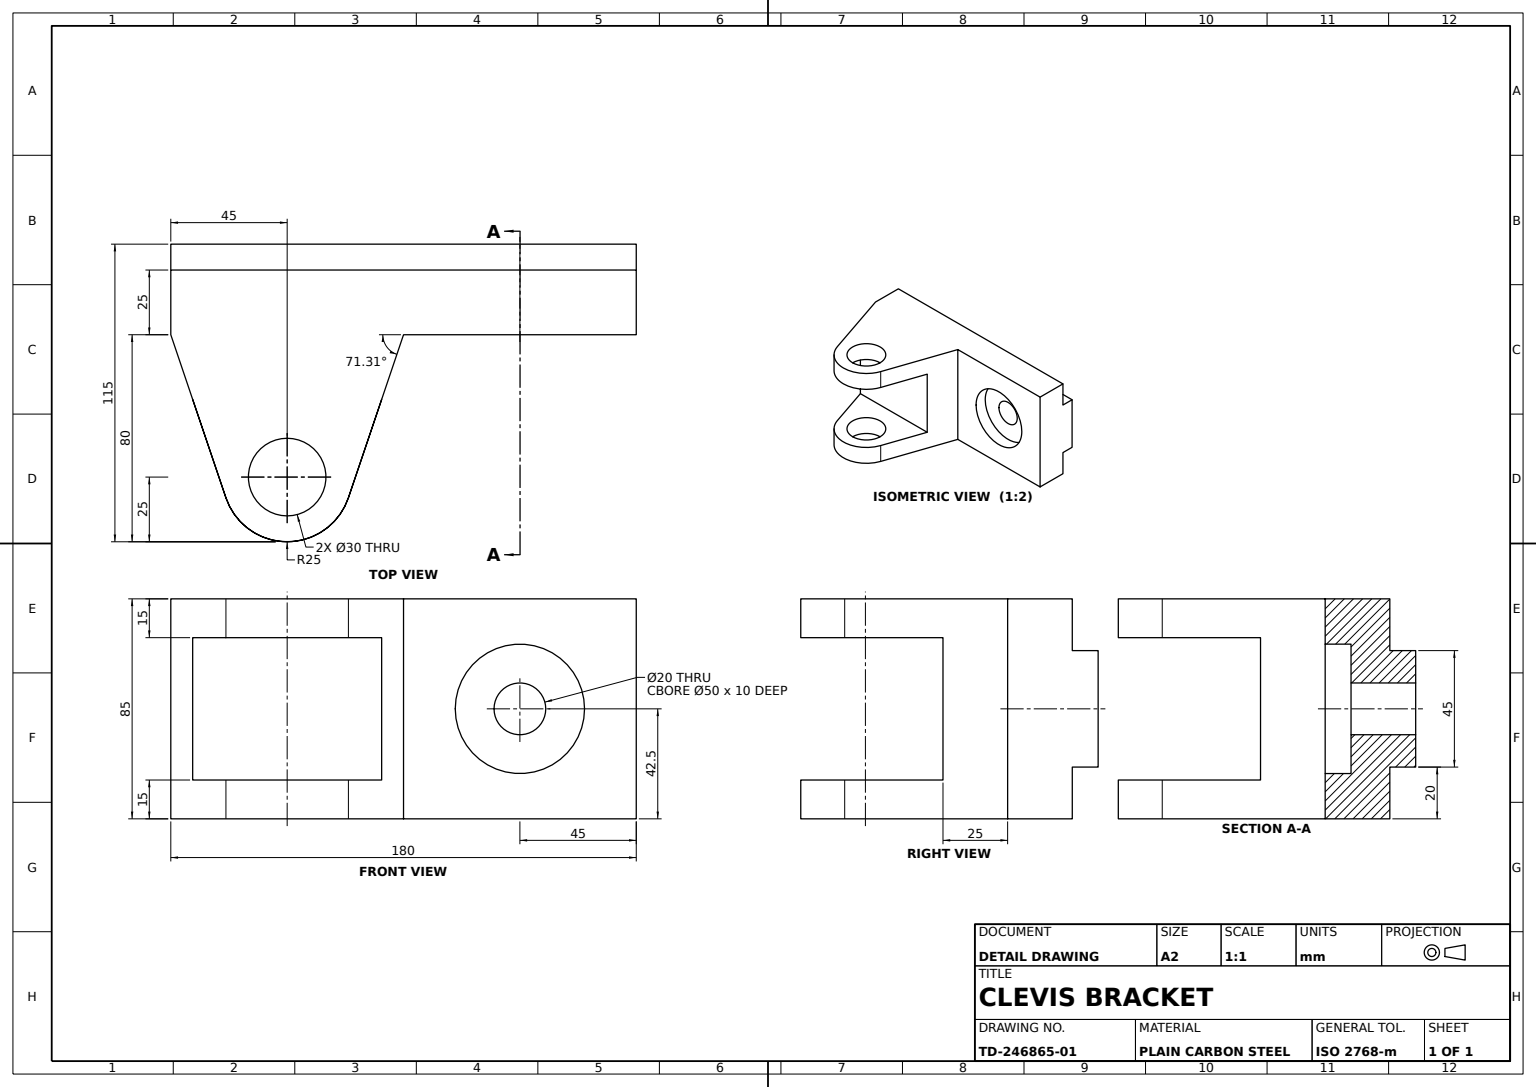
SolidWorks part; units mm, degrees
material "Plain Carbon Steel"
ref_plane "Front Plane" through (0, 0, 0) normal (0, 0, 1) x (1, 0, 0)
ref_plane "Top Plane" through (0, 0, 0) normal (0, 1, 0) x (1, 0, 0)
ref_plane "Right Plane" through (0, 0, 0) normal (1, 0, 0) x (0, 0, -1)
sketch "Base Plate Sketch" plane through (0, 0, 0) normal (0, 0, 1) x (1, 0, 0)
  line L0 (-210.1104, 0) -> (185.8735, 0) construction
  line L1 (0, 117.6004) -> (0, -132.2791) construction
  line L3 (-90, -42.5) -> (90, -42.5)
  line L4 (-90, -42.5) -> (-90, 42.5)
  line L5 (-90, 42.5) -> (90, 42.5)
  line L6 (90, -42.5) -> (90, 42.5)
  line L7 (-90, -42.5) -> (90, 42.5) construction
  line L8 (-90, 42.5) -> (90, -42.5) construction
  point P5 (0, 0)
  dimension "D1" = 85
  dimension "D2" = 180
extrude "Base Plate" add sketch "Base Plate Sketch" along normal blind 25
sketch "Counterbore Sketch" plane through (0, 0, 25) normal (0, 0, 1) x (1, 0, 0)
  line L0 (-0.6032, 58.2808) -> (0.6771, -65.4214) construction
  line L1 (0, 0) -> (90, 0) construction
  line L2 (90, -42.5) -> (90, 42.5) construction
  circle A0 centre (45, 0) radius 25
  dimension "D1" = 50
  dimension "D2" = 90.593
extrude "Counterbore Ø50" cut sketch "Counterbore Sketch" against normal blind 10
sketch "Through Hole Sketch" plane through (0, 0, 15) normal (0, 0, 1) x (1, 0, 0)
  circle A0 centre (45, 0) radius 10
  dimension "D1" = 20
extrude "Through Hole Ø20" cut sketch "Through Hole Sketch" against normal blind 20
sketch "Back Key Sketch" plane through (-90, 0, 0) normal (-1, 0, 0) x (0, 0, 1)
  line L0 (-56.1087, 0) -> (65.6103, 0) construction
  line L1 (0, 42.5) -> (0, -42.5) construction
  line L2 (0, 22.5) -> (-10, 22.5)
  line L3 (0, 22.5) -> (0, -22.5)
  line L4 (0, -22.5) -> (-10, -22.5)
  line L5 (-10, 22.5) -> (-10, -22.5)
  dimension "D1" = 45
  dimension "D2" = 10
extrude "Back Key" add sketch "Back Key Sketch" against normal through all
sketch "Key Relief Sketch" plane through (0, 0, 0) normal (0, 0, 1) x (1, 0, 0)
  circle A1 centre (45, 0) radius 10
  circle A2 centre (45, 0) radius 10
  dimension "D1" = 0
extrude "Key Relief Cut" cut sketch "Key Relief Sketch" against normal through all
sketch "Upper Lug Sketch" plane through (0, -42.5, 0) normal (0, -1, 0) x (1, 0, 0)
  line L0 (0, 0) -> (0, 65.1444) construction
  line L1 (-45, 0) -> (-45, 80) construction
  line L2 (-68.6814, 88.012) -> (-90, 25)
  line L3 (-21.3186, 88.012) -> (0, 25)
  line L4 (-90, 0) -> (90, 0)
  line L5 (90, 0) -> (90, 25)
  line L6 (90, 25) -> (-90, 25)
  line L7 (-90, 25) -> (-90, 0)
  line L10 (0, 25) -> (-90, 25)
  circle A0 centre (-45, 80) radius 15
  arc A1 (-21.3186, 88.012) -> (-68.6814, 88.012) centre (-45, 80) ccw
  dimension "D4" = 30
  dimension "D5" = 50
  dimension "D3" = 80
  dimension "D1" = 0
extrude "Upper Lug" add sketch "Upper Lug Sketch" against normal blind 15
sketch "Lower Lug Sketch" plane through (0, 42.5, 0) normal (0, 1, 0) x (1, 0, 0)
  line L0 (-45, -25) -> (-45, -80) construction
  line L1 (-90, -25) -> (-90, 0) construction
  line L2 (-90, -25) -> (-68.6814, -88.012)
  line L3 (0, -25) -> (-21.3186, -88.012)
  line L4 (90, 0) -> (-90, 0)
  line L5 (-90, 0) -> (-90, -25)
  line L6 (-90, -25) -> (90, -25)
  line L7 (90, -25) -> (90, 0)
  line L10 (-90, -25) -> (0, -25)
  circle A0 centre (-45, -80) radius 15
  arc A1 (-68.6814, -88.012) -> (-21.3186, -88.012) centre (-45, -80) ccw
  dimension "D4" = 30
  dimension "D5" = 50
  dimension "D2" = 21.3186
  dimension "D3" = 55
  dimension "D1" = 0
extrude "Lower Lug" add sketch "Lower Lug Sketch" against normal blind 15
sketch "Lug Web Sketch" plane through (0, 0, 25) normal (0, 0, 1) x (1, 0, 0)
  line L0 (0, 27.5) -> (0, -27.5)
  line L8 (90, 42.5) -> (0, 42.5)
  line L9 (0, 42.5) -> (0, 27.5)
  line L10 (0, 27.5) -> (-90, 27.5)
  line L11 (-90, 27.5) -> (-90, -27.5)
  line L12 (-90, -27.5) -> (0, -27.5)
  line L13 (0, -27.5) -> (0, -42.5)
  line L14 (0, -42.5) -> (90, -42.5)
  line L15 (90, -42.5) -> (90, 42.5)
  line L18 (0, 27.5) -> (-90, 27.5)
  line L19 (-90, 27.5) -> (-90, -27.5)
  line L20 (-90, -27.5) -> (0, -27.5)
  dimension "D1" = 0
extrude "Lug Web" add sketch "Lug Web Sketch" along normal blind 25
sketch "Web Cut A Sketch" plane through (0, 27.5, 0) normal (0, 1, 0) x (1, 0, 0)
  line L3 (0, -25) -> (-8.4582, -50)
  line L4 (-8.4582, -50) -> (0, -50)
  line L5 (0, -50) -> (0, -25)
  line L6 (0, -25) -> (-8.4582, -50)
  line L7 (-8.4582, -50) -> (0, -50)
  line L8 (0, -50) -> (0, -25)
  dimension "D1" = 0
extrude "Web Cut A" cut sketch "Web Cut A Sketch" against normal through all
sketch "Web Cut B Sketch" plane through (0, -27.5, 0) normal (0, -1, 0) x (1, 0, 0)
  line L3 (-90, 25) -> (-81.5418, 50)
  line L4 (-81.5418, 50) -> (-90, 50)
  line L5 (-90, 50) -> (-90, 25)
  line L6 (-90, 25) -> (-81.5418, 50)
  line L7 (-81.5418, 50) -> (-90, 50)
  line L8 (-90, 50) -> (-90, 25)
  dimension "D1" = 0
extrude "Web Cut B" cut sketch "Web Cut B Sketch" against normal through all
